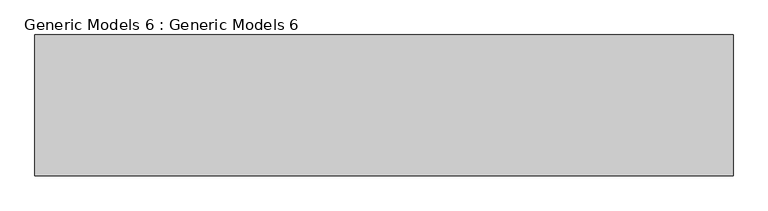
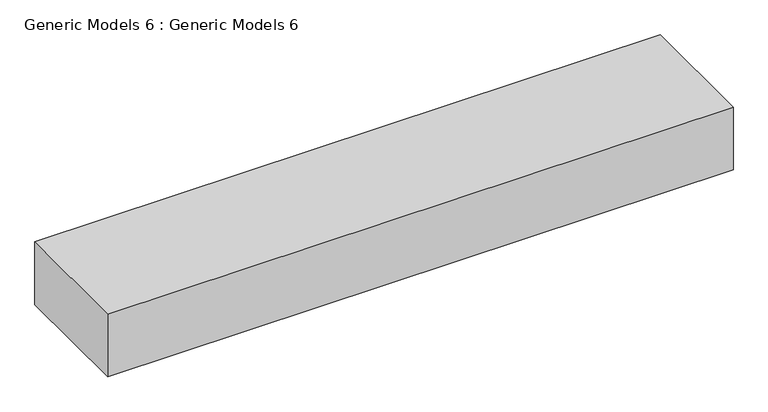
"""IFC4 building model written with IfcOpenShell, lengths in millimetres: proxy geometry, Generic Models 6 : Generic Models 6."""

from ifc_helpers import new_model, si_unit, frame, origin, place, context, project, spatial, polyline, outline, extrude, source, transform, mapped, element, save


def generic_models_6_generic_models_6_f1c04d34(model_context):
    return source(origin(), model_context, "Body", "SweptSolid", [
        extrude(outline(polyline([(-8605.1750786, -14078.0808221), (-8605.1750786, -15692.2933703), (-16607.9505427, -15692.2933703), (-16607.9505427, -14078.0808221), (-8605.1750786, -14078.0808221)])), frame((0.0, 0.0, 5783.5856694), z_axis=(0.0, 0.0, 1.0), x_axis=(1.0, 0.0, 0.0)), (0.0, 0.0, 1.0), 845.8143306),
    ])


if __name__ == "__main__":
    model = new_model("IFC4")
    model_context = context("Model", 3, world=origin())
    ifc_project = project(units=[si_unit("LENGTHUNIT", "METRE", prefix="MILLI")], contexts=[model_context])
    site = spatial("IfcSite", under=ifc_project)
    building = spatial("IfcBuilding", under=site)
    placement = place(None, origin())
    generic_models_6_generic_models_6_shape = generic_models_6_generic_models_6_f1c04d34(model_context)
    element("IfcBuildingElementProxy", 1, Name="Generic Models 6 : Generic Models 6", ObjectType="Generic Models 6 : Generic Models 6", at=placement, inside=building, context=model_context, shape_type="MappedRepresentation", body=[
        mapped(generic_models_6_generic_models_6_shape, transform((0.0, 0.0, 0.0), x_axis=(1.0, 0.0, 0.0), y_axis=(0.0, 1.0, 0.0), z_axis=(0.0, 0.0, 1.0))),
    ])
    save(model, "model.ifc")
